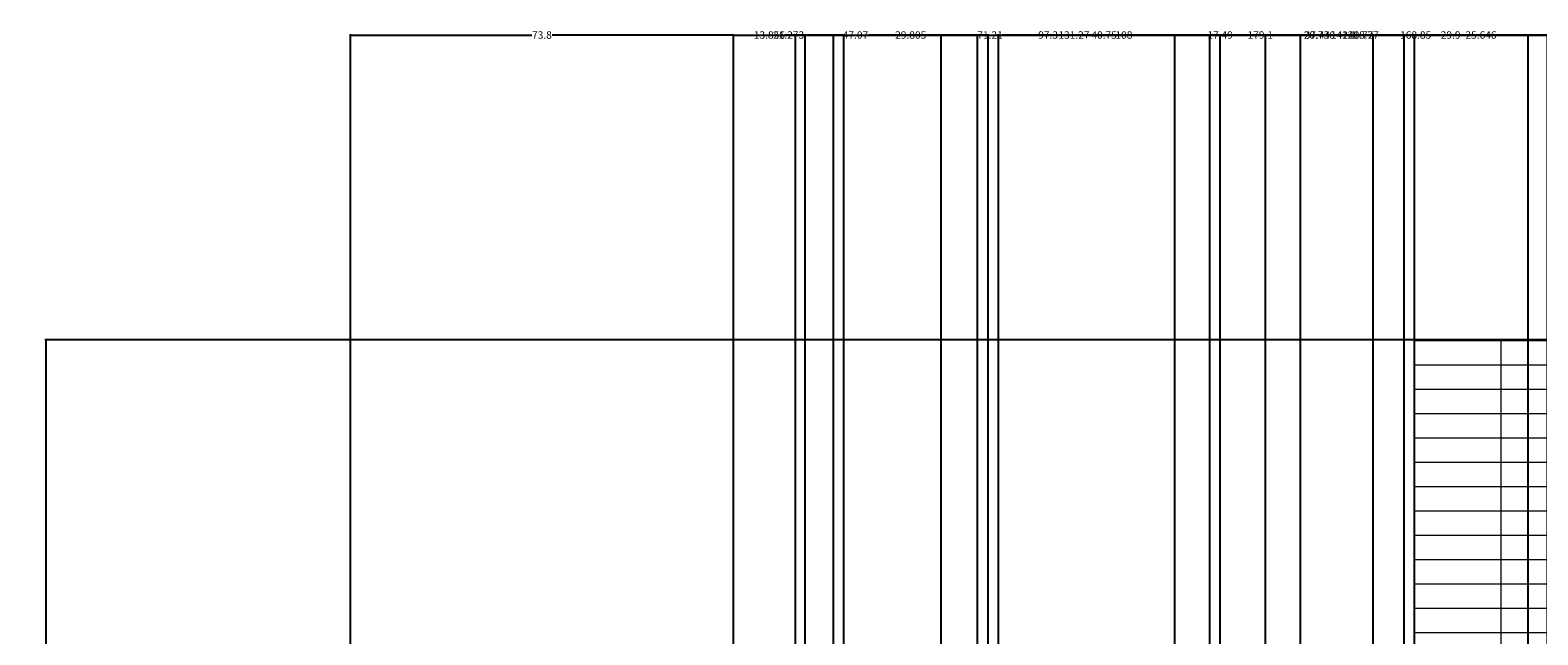
# Model space of a CAD drawing. Units: inches. Extents: x 241 to 943, y 109 to 1396.
# Tile 25 of 34: x 241 to 532, y 1279 to 1396. Entities that reach past the tile are written whole.
import ezdxf

# ---------------------------------------------------------------- set-up
doc = ezdxf.new("R2010")
doc.units = ezdxf.units.IN
doc.header["$MEASUREMENT"] = 0
for name, color, linetype, lineweight in [('A-ANNO-DIMS', 2, 'Continuous', 18), ('A-ELEV', 7, 'Continuous', 25), ('A-WALL-PATT', 8, 'Continuous', 13)]:
    doc.layers.add(name, color=color, linetype=linetype, lineweight=lineweight)
doc.styles.get("Standard").update_dxf_attribs({"font": 'arial.ttf'})
doc.dimstyles.get("Standard").update_dxf_attribs({"dimtxt": 1.4375, "dimasz": 0.18, "dimexe": 0.18, "dimexo": 0.0625, "dimgap": 0.09, "dimtad": 0, "dimtih": 1, "dimtoh": 1, "dimdec": 4, "dimzin": 0, "dimdsep": 46, "dimlunit": 4, "dimtxsty": 'Standard', "dimcen": 0.09, "dimadec": 0, "dimazin": 0, "dimtfac": 1, "dimtdec": 4, "dimtofl": 0, "dimtmove": 0, "dimatfit": 3, "dimfxl": 1, "dimtolj": 1, "dimtzin": 0, "dimarcsym": 0})

# ---------------------------------------------------------------- blocks, each defined once
blk = doc.blocks.new('*D5')
at = {"layer": 'A-ANNO-DIMS', "color": 0, "lineweight": -2, "transparency": 16777216}
for p, q in [((303.24, 177.8), (303.24, 1395.05)), ((377.04, 177.76), (377.04, 1395.05)), ((303.42, 1394.87), (338.18, 1394.87)), ((376.86, 1394.87), (342.09, 1394.87))]:
    blk.add_line(p, q, dxfattribs=at)
at = {"layer": 'A-ANNO-DIMS', "color": 0, "transparency": 16777216}
for points in [[(303.42, 1394.9), (303.42, 1394.84), (303.24, 1394.87)], [(376.86, 1394.9), (376.86, 1394.84), (377.04, 1394.87)]]:
    blk.add_solid(points, dxfattribs=at)
at = {"layer": 'Defpoints', "color": 0, "transparency": 16777216}
for p in [(377.04, 1394.87), (303.24, 177.74), (377.04, 177.7)]:
    blk.add_point(p, dxfattribs=at)
at = {"layer": 'A-ANNO-DIMS', "color": 0, "transparency": 16777216, "insert": (340.14, 1394.87), "char_height": 1.438, "attachment_point": 5}
blk.add_mtext('\\A1;73.8', dxfattribs=at)
blk = doc.blocks.new('*D7')
at = {"layer": 'A-ANNO-DIMS', "color": 0, "lineweight": -2, "transparency": 16777216}
for p, q in [((508.24, 1336.12), (244.31, 1336.12)), ((244.49, 1335.94), (244.49, 753.25)), ((244.49, 168.92), (244.49, 751.6)), ((303.17, 168.74), (244.31, 168.74))]:
    blk.add_line(p, q, dxfattribs=at)
at = {"layer": 'A-ANNO-DIMS', "color": 0, "transparency": 16777216}
for points in [[(244.46, 1335.94), (244.52, 1335.94), (244.49, 1336.12)], [(244.46, 168.92), (244.52, 168.92), (244.49, 168.74)]]:
    blk.add_solid(points, dxfattribs=at)
at = {"layer": 'Defpoints', "color": 0, "transparency": 16777216}
for p in [(244.49, 1336.12), (508.31, 1336.12), (303.24, 168.74)]:
    blk.add_point(p, dxfattribs=at)
at = {"layer": 'A-ANNO-DIMS', "color": 0, "transparency": 16777216, "insert": (244.49, 752.43), "char_height": 1.438, "attachment_point": 5}
blk.add_mtext('\\A1;1167.4', dxfattribs=at)
blk = doc.blocks.new('*D8')
at = {"layer": 'A-ANNO-DIMS', "color": 0, "lineweight": -2, "transparency": 16777216}
for p, q in [((377.04, 396.94), (377.04, 1395.05)), ((390.89, 384.24), (390.89, 1395.05)), ((377.22, 1394.87), (380.96, 1394.87)), ((390.71, 1394.87), (386.97, 1394.87))]:
    blk.add_line(p, q, dxfattribs=at)
at = {"layer": 'A-ANNO-DIMS', "color": 0, "transparency": 16777216}
for points in [[(377.22, 1394.9), (377.22, 1394.84), (377.04, 1394.87)], [(390.71, 1394.9), (390.71, 1394.84), (390.89, 1394.87)]]:
    blk.add_solid(points, dxfattribs=at)
at = {"layer": 'Defpoints', "color": 0, "transparency": 16777216}
for p in [(390.89, 1394.87), (377.04, 396.88), (390.89, 384.18)]:
    blk.add_point(p, dxfattribs=at)
at = {"layer": 'A-ANNO-DIMS', "color": 0, "transparency": 16777216, "insert": (383.97, 1394.87), "char_height": 1.438, "attachment_point": 5}
blk.add_mtext('\\A1;13.856', dxfattribs=at)
blk = doc.blocks.new('*D9')
at = {"layer": 'A-ANNO-DIMS', "color": 0, "lineweight": -2, "transparency": 16777216}
for p, q in [((390.89, 384.24), (390.89, 1395.05)), ((462.11, 384.24), (462.11, 1395.05)), ((391.07, 1394.87), (424.13, 1394.87)), ((461.93, 1394.87), (428.87, 1394.87))]:
    blk.add_line(p, q, dxfattribs=at)
at = {"layer": 'A-ANNO-DIMS', "color": 0, "transparency": 16777216}
for points in [[(391.07, 1394.9), (391.07, 1394.84), (390.89, 1394.87)], [(461.93, 1394.9), (461.93, 1394.84), (462.11, 1394.87)]]:
    blk.add_solid(points, dxfattribs=at)
at = {"layer": 'Defpoints', "color": 0, "transparency": 16777216}
for p in [(462.11, 1394.87), (390.89, 384.18), (462.11, 384.18)]:
    blk.add_point(p, dxfattribs=at)
at = {"layer": 'A-ANNO-DIMS', "color": 0, "transparency": 16777216, "insert": (426.5, 1394.87), "char_height": 1.438, "attachment_point": 5}
blk.add_mtext('\\A1;71.21', dxfattribs=at)
blk = doc.blocks.new('*D10')
at = {"layer": 'A-ANNO-DIMS', "color": 0, "lineweight": -2, "transparency": 16777216}
for p, q in [((462.11, 384.24), (462.11, 1395.05)), ((479.6, 384.24), (479.6, 1395.05)), ((462.29, 1394.87), (468.4, 1394.87)), ((479.42, 1394.87), (473.3, 1394.87))]:
    blk.add_line(p, q, dxfattribs=at)
at = {"layer": 'A-ANNO-DIMS', "color": 0, "transparency": 16777216}
for points in [[(462.29, 1394.9), (462.29, 1394.84), (462.11, 1394.87)], [(479.42, 1394.9), (479.42, 1394.84), (479.6, 1394.87)]]:
    blk.add_solid(points, dxfattribs=at)
at = {"layer": 'Defpoints', "color": 0, "transparency": 16777216}
for p in [(479.6, 1394.87), (462.11, 384.18), (479.6, 384.18)]:
    blk.add_point(p, dxfattribs=at)
at = {"layer": 'A-ANNO-DIMS', "color": 0, "transparency": 16777216, "insert": (470.85, 1394.87), "char_height": 1.438, "attachment_point": 5}
blk.add_mtext('\\A1;17.49', dxfattribs=at)
blk = doc.blocks.new('*D11')
at = {"layer": 'A-ANNO-DIMS', "color": 0, "lineweight": -2, "transparency": 16777216}
for p, q in [((500.33, 384.24), (500.33, 1395.05)), ((530.23, 384.24), (530.23, 1395.05)), ((500.51, 1394.87), (513.31, 1394.87)), ((530.05, 1394.87), (517.25, 1394.87))]:
    blk.add_line(p, q, dxfattribs=at)
at = {"layer": 'A-ANNO-DIMS', "color": 0, "transparency": 16777216}
for points in [[(500.51, 1394.9), (500.51, 1394.84), (500.33, 1394.87)], [(530.05, 1394.9), (530.05, 1394.84), (530.23, 1394.87)]]:
    blk.add_solid(points, dxfattribs=at)
at = {"layer": 'Defpoints', "color": 0, "transparency": 16777216}
for p in [(530.23, 1394.87), (500.33, 384.18), (530.23, 384.18)]:
    blk.add_point(p, dxfattribs=at)
at = {"layer": 'A-ANNO-DIMS', "color": 0, "transparency": 16777216, "insert": (515.28, 1394.87), "char_height": 1.438, "attachment_point": 5}
blk.add_mtext('\\A1;29.9', dxfattribs=at)
blk = doc.blocks.new('*D12')
at = {"layer": 'A-ANNO-DIMS', "color": 0, "lineweight": -2, "transparency": 16777216}
for p, q in [((530.23, 384.24), (530.23, 1395.05)), ((650.91, 384.24), (650.91, 1395.05)), ((530.41, 1394.87), (587.56, 1394.87)), ((650.73, 1394.87), (593.58, 1394.87))]:
    blk.add_line(p, q, dxfattribs=at)
at = {"layer": 'A-ANNO-DIMS', "color": 0, "transparency": 16777216}
for points in [[(530.41, 1394.9), (530.41, 1394.84), (530.23, 1394.87)], [(650.73, 1394.9), (650.73, 1394.84), (650.91, 1394.87)]]:
    blk.add_solid(points, dxfattribs=at)
at = {"layer": 'Defpoints', "color": 0, "transparency": 16777216}
for p in [(650.91, 1394.87), (530.23, 384.18), (650.91, 384.18)]:
    blk.add_point(p, dxfattribs=at)
at = {"layer": 'A-ANNO-DIMS', "color": 0, "transparency": 16777216, "insert": (590.57, 1394.87), "char_height": 1.438, "attachment_point": 5}
blk.add_mtext('\\A1;120.68', dxfattribs=at)
blk = doc.blocks.new('*D17')
at = {"layer": 'A-ANNO-DIMS', "color": 0, "lineweight": -2, "transparency": 16777216}
for p, q in [((377.04, 1275.98), (377.04, 1395.05)), ((508.31, 1275.98), (508.31, 1395.05)), ((377.22, 1394.87), (439.67, 1394.87)), ((508.13, 1394.87), (445.68, 1394.87))]:
    blk.add_line(p, q, dxfattribs=at)
at = {"layer": 'A-ANNO-DIMS', "color": 0, "transparency": 16777216}
for points in [[(377.22, 1394.9), (377.22, 1394.84), (377.04, 1394.87)], [(508.13, 1394.9), (508.13, 1394.84), (508.31, 1394.87)]]:
    blk.add_solid(points, dxfattribs=at)
at = {"layer": 'Defpoints', "color": 0, "transparency": 16777216}
for p in [(508.31, 1394.87), (377.04, 1275.91), (508.31, 1275.91)]:
    blk.add_point(p, dxfattribs=at)
at = {"layer": 'A-ANNO-DIMS', "color": 0, "transparency": 16777216, "insert": (442.67, 1394.87), "char_height": 1.438, "attachment_point": 5}
blk.add_mtext('\\A1;131.27', dxfattribs=at)
blk = doc.blocks.new('*D18')
at = {"layer": 'A-ANNO-DIMS', "color": 0, "lineweight": -2, "transparency": 16777216}
for p, q in [((508.31, 1336.18), (508.31, 1395.05)), ((747.76, 1336.18), (747.76, 1395.05)), ((508.49, 1394.87), (624.94, 1394.87)), ((747.58, 1394.87), (631.12, 1394.87))]:
    blk.add_line(p, q, dxfattribs=at)
at = {"layer": 'A-ANNO-DIMS', "color": 0, "transparency": 16777216}
for points in [[(508.49, 1394.9), (508.49, 1394.84), (508.31, 1394.87)], [(747.58, 1394.9), (747.58, 1394.84), (747.76, 1394.87)]]:
    blk.add_solid(points, dxfattribs=at)
at = {"layer": 'Defpoints', "color": 0, "transparency": 16777216}
for p in [(747.76, 1394.87), (508.31, 1336.12), (747.76, 1336.12)]:
    blk.add_point(p, dxfattribs=at)
at = {"layer": 'A-ANNO-DIMS', "color": 0, "transparency": 16777216, "insert": (628.03, 1394.87), "char_height": 1.438, "attachment_point": 5}
blk.add_mtext('\\A1;239.45', dxfattribs=at)
blk = doc.blocks.new('*D57')
at = {"layer": 'A-ANNO-DIMS', "color": 0, "lineweight": -2, "transparency": 16777216}
for p, q in [((508.31, 1070.92), (508.31, 1395.05)), ((533.95, 1108.23), (533.95, 1395.05)), ((508.49, 1394.87), (518.04, 1394.87)), ((533.77, 1394.87), (524.21, 1394.87))]:
    blk.add_line(p, q, dxfattribs=at)
at = {"layer": 'A-ANNO-DIMS', "color": 0, "transparency": 16777216}
for points in [[(508.49, 1394.9), (508.49, 1394.84), (508.31, 1394.87)], [(533.77, 1394.9), (533.77, 1394.84), (533.95, 1394.87)]]:
    blk.add_solid(points, dxfattribs=at)
at = {"layer": 'Defpoints', "color": 0, "transparency": 16777216}
for p in [(533.95, 1394.87), (533.95, 1108.17), (508.31, 1070.85)]:
    blk.add_point(p, dxfattribs=at)
at = {"layer": 'A-ANNO-DIMS', "color": 0, "transparency": 16777216, "insert": (521.13, 1394.87), "char_height": 1.438, "attachment_point": 5}
blk.add_mtext('\\A1;25.646', dxfattribs=at)
blk = doc.blocks.new('*D59')
at = {"layer": 'A-ANNO-DIMS', "color": 0, "lineweight": -2, "transparency": 16777216}
for p, q in [((398.31, 1175.6), (398.31, 1395.05)), ((506.31, 1175.6), (506.31, 1395.05)), ((398.49, 1394.87), (450.7, 1394.87)), ((506.13, 1394.87), (453.92, 1394.87))]:
    blk.add_line(p, q, dxfattribs=at)
at = {"layer": 'A-ANNO-DIMS', "color": 0, "transparency": 16777216}
for points in [[(398.49, 1394.9), (398.49, 1394.84), (398.31, 1394.87)], [(506.13, 1394.9), (506.13, 1394.84), (506.31, 1394.87)]]:
    blk.add_solid(points, dxfattribs=at)
at = {"layer": 'Defpoints', "color": 0, "transparency": 16777216}
for p in [(506.31, 1394.87), (398.31, 1175.54), (506.31, 1175.54)]:
    blk.add_point(p, dxfattribs=at)
at = {"layer": 'A-ANNO-DIMS', "color": 0, "transparency": 16777216, "insert": (452.31, 1394.87), "char_height": 1.438, "attachment_point": 5}
blk.add_mtext('\\A1;108', dxfattribs=at)
blk = doc.blocks.new('*D60')
at = {"layer": 'A-ANNO-DIMS', "color": 0, "lineweight": -2, "transparency": 16777216}
for p, q in [((377.04, 1177.6), (377.04, 1395.05)), ((398.31, 1175.6), (398.31, 1395.05)), ((377.22, 1394.87), (384.59, 1394.87)), ((398.13, 1394.87), (390.76, 1394.87))]:
    blk.add_line(p, q, dxfattribs=at)
at = {"layer": 'A-ANNO-DIMS', "color": 0, "transparency": 16777216}
for points in [[(377.22, 1394.9), (377.22, 1394.84), (377.04, 1394.87)], [(398.13, 1394.9), (398.13, 1394.84), (398.31, 1394.87)]]:
    blk.add_solid(points, dxfattribs=at)
at = {"layer": 'Defpoints', "color": 0, "transparency": 16777216}
for p in [(398.31, 1394.87), (377.04, 1177.54), (398.31, 1175.54)]:
    blk.add_point(p, dxfattribs=at)
at = {"layer": 'A-ANNO-DIMS', "color": 0, "transparency": 16777216, "insert": (387.68, 1394.87), "char_height": 1.438, "attachment_point": 5}
blk.add_mtext('\\A1;21.273', dxfattribs=at)
blk = doc.blocks.new('*D61')
at = {"layer": 'A-ANNO-DIMS', "color": 0, "lineweight": -2, "transparency": 16777216}
for p, q in [((377.04, 400.89), (377.04, 1395.05)), ((424.11, 568.89), (424.11, 1395.05)), ((377.22, 1394.87), (398.03, 1394.87)), ((423.93, 1394.87), (403.12, 1394.87))]:
    blk.add_line(p, q, dxfattribs=at)
at = {"layer": 'A-ANNO-DIMS', "color": 0, "transparency": 16777216}
for points in [[(377.22, 1394.9), (377.22, 1394.84), (377.04, 1394.87)], [(423.93, 1394.9), (423.93, 1394.84), (424.11, 1394.87)]]:
    blk.add_solid(points, dxfattribs=at)
at = {"layer": 'Defpoints', "color": 0, "transparency": 16777216}
for p in [(424.11, 1394.87), (424.11, 568.83), (377.04, 400.83)]:
    blk.add_point(p, dxfattribs=at)
at = {"layer": 'A-ANNO-DIMS', "color": 0, "transparency": 16777216, "insert": (400.57, 1394.87), "char_height": 1.438, "attachment_point": 5}
blk.add_mtext('\\A1;47.07', dxfattribs=at)
blk = doc.blocks.new('*D62')
at = {"layer": 'A-ANNO-DIMS', "color": 0, "lineweight": -2, "transparency": 16777216}
for p, q in [((424.11, 568.89), (424.11, 1395.05)), ((565.2, 568.89), (565.2, 1395.05)), ((424.29, 1394.87), (492.35, 1394.87)), ((565.02, 1394.87), (496.96, 1394.87))]:
    blk.add_line(p, q, dxfattribs=at)
at = {"layer": 'A-ANNO-DIMS', "color": 0, "transparency": 16777216}
for points in [[(424.29, 1394.9), (424.29, 1394.84), (424.11, 1394.87)], [(565.02, 1394.9), (565.02, 1394.84), (565.2, 1394.87)]]:
    blk.add_solid(points, dxfattribs=at)
at = {"layer": 'Defpoints', "color": 0, "transparency": 16777216}
for p in [(565.2, 1394.87), (424.11, 568.83), (565.2, 568.83)]:
    blk.add_point(p, dxfattribs=at)
at = {"layer": 'A-ANNO-DIMS', "color": 0, "transparency": 16777216, "insert": (494.66, 1394.87), "char_height": 1.438, "attachment_point": 5}
blk.add_mtext('\\A1;141.1', dxfattribs=at)
blk = doc.blocks.new('*D65')
at = {"layer": 'A-ANNO-DIMS', "color": 0, "lineweight": -2, "transparency": 16777216}
for p, q in [((424.11, 700.85), (424.11, 1395.05)), ((592.95, 700.85), (592.95, 1395.05)), ((424.29, 1394.87), (505.52, 1394.87)), ((592.77, 1394.87), (511.54, 1394.87))]:
    blk.add_line(p, q, dxfattribs=at)
at = {"layer": 'A-ANNO-DIMS', "color": 0, "transparency": 16777216}
for points in [[(424.29, 1394.9), (424.29, 1394.84), (424.11, 1394.87)], [(592.77, 1394.9), (592.77, 1394.84), (592.95, 1394.87)]]:
    blk.add_solid(points, dxfattribs=at)
at = {"layer": 'Defpoints', "color": 0, "transparency": 16777216}
for p in [(592.95, 1394.87), (424.11, 700.79), (592.95, 700.79)]:
    blk.add_point(p, dxfattribs=at)
at = {"layer": 'A-ANNO-DIMS', "color": 0, "transparency": 16777216, "insert": (508.53, 1394.87), "char_height": 1.438, "attachment_point": 5}
blk.add_mtext('\\A1;168.85', dxfattribs=at)
blk = doc.blocks.new('*D67')
at = {"layer": 'A-ANNO-DIMS', "color": 0, "lineweight": -2, "transparency": 16777216}
for p, q in [((389.04, 773.55), (389.04, 1395.05)), ((607.82, 773.55), (607.82, 1395.05)), ((389.22, 1394.87), (495.34, 1394.87)), ((607.64, 1394.87), (501.52, 1394.87))]:
    blk.add_line(p, q, dxfattribs=at)
at = {"layer": 'A-ANNO-DIMS', "color": 0, "transparency": 16777216}
for points in [[(389.22, 1394.9), (389.22, 1394.84), (389.04, 1394.87)], [(607.64, 1394.9), (607.64, 1394.84), (607.82, 1394.87)]]:
    blk.add_solid(points, dxfattribs=at)
at = {"layer": 'Defpoints', "color": 0, "transparency": 16777216}
for p in [(607.82, 1394.87), (389.04, 773.49), (607.82, 773.49)]:
    blk.add_point(p, dxfattribs=at)
at = {"layer": 'A-ANNO-DIMS', "color": 0, "transparency": 16777216, "insert": (498.43, 1394.87), "char_height": 1.438, "attachment_point": 5}
blk.add_mtext('\\A1;218.77', dxfattribs=at)
blk = doc.blocks.new('*D69')
at = {"layer": 'A-ANNO-DIMS', "color": 0, "lineweight": -2, "transparency": 16777216}
for p, q in [((389.04, 941.55), (389.04, 1395.05)), ((568.13, 941.55), (568.13, 1395.05)), ((389.22, 1394.87), (476.28, 1394.87)), ((567.95, 1394.87), (480.9, 1394.87))]:
    blk.add_line(p, q, dxfattribs=at)
at = {"layer": 'A-ANNO-DIMS', "color": 0, "transparency": 16777216}
for points in [[(389.22, 1394.9), (389.22, 1394.84), (389.04, 1394.87)], [(567.95, 1394.9), (567.95, 1394.84), (568.13, 1394.87)]]:
    blk.add_solid(points, dxfattribs=at)
at = {"layer": 'Defpoints', "color": 0, "transparency": 16777216}
for p in [(568.13, 1394.87), (389.04, 941.49), (568.13, 941.49)]:
    blk.add_point(p, dxfattribs=at)
at = {"layer": 'A-ANNO-DIMS', "color": 0, "transparency": 16777216, "insert": (478.59, 1394.87), "char_height": 1.438, "attachment_point": 5}
blk.add_mtext('\\A1;179.1', dxfattribs=at)
blk = doc.blocks.new('*D72')
at = {"layer": 'A-ANNO-DIMS', "color": 0, "lineweight": -2, "transparency": 16777216}
for p, q in [((389.04, 1109.55), (389.04, 1395.05)), ((486.34, 1109.55), (486.34, 1395.05)), ((389.22, 1394.87), (435.74, 1394.87)), ((486.16, 1394.87), (439.65, 1394.87))]:
    blk.add_line(p, q, dxfattribs=at)
at = {"layer": 'A-ANNO-DIMS', "color": 0, "transparency": 16777216}
for points in [[(389.22, 1394.9), (389.22, 1394.84), (389.04, 1394.87)], [(486.16, 1394.9), (486.16, 1394.84), (486.34, 1394.87)]]:
    blk.add_solid(points, dxfattribs=at)
at = {"layer": 'Defpoints', "color": 0, "transparency": 16777216}
for p in [(486.34, 1394.87), (389.04, 1109.49), (486.34, 1109.49)]:
    blk.add_point(p, dxfattribs=at)
at = {"layer": 'A-ANNO-DIMS', "color": 0, "transparency": 16777216, "insert": (437.69, 1394.87), "char_height": 1.438, "attachment_point": 5}
blk.add_mtext('\\A1;97.3', dxfattribs=at)
blk = doc.blocks.new('*D79')
at = {"layer": 'A-ANNO-DIMS', "color": 0, "lineweight": -2, "transparency": 16777216}
for p, q in [((479.6, 384.24), (479.6, 1395.05)), ((500.33, 384.24), (500.33, 1395.05)), ((479.78, 1394.87), (486.88, 1394.87)), ((500.15, 1394.87), (493.05, 1394.87))]:
    blk.add_line(p, q, dxfattribs=at)
at = {"layer": 'A-ANNO-DIMS', "color": 0, "transparency": 16777216}
for points in [[(479.78, 1394.9), (479.78, 1394.84), (479.6, 1394.87)], [(500.15, 1394.9), (500.15, 1394.84), (500.33, 1394.87)]]:
    blk.add_solid(points, dxfattribs=at)
at = {"layer": 'Defpoints', "color": 0, "transparency": 16777216}
for p in [(500.33, 1394.87), (479.6, 384.18), (500.33, 384.18)]:
    blk.add_point(p, dxfattribs=at)
at = {"layer": 'A-ANNO-DIMS', "color": 0, "transparency": 16777216, "insert": (489.96, 1394.87), "char_height": 1.438, "attachment_point": 5}
blk.add_mtext('\\A1;20.736', dxfattribs=at)
blk = doc.blocks.new('*D89')
at = {"layer": 'A-ANNO-DIMS', "color": 0, "lineweight": -2, "transparency": 16777216}
for p, q in [((377.04, 841.6), (377.04, 1395.05)), ((617.76, 841.6), (617.76, 1395.05)), ((377.22, 1394.87), (494.32, 1394.87)), ((617.58, 1394.87), (500.48, 1394.87))]:
    blk.add_line(p, q, dxfattribs=at)
at = {"layer": 'A-ANNO-DIMS', "color": 0, "transparency": 16777216}
for points in [[(377.22, 1394.9), (377.22, 1394.84), (377.04, 1394.87)], [(617.58, 1394.9), (617.58, 1394.84), (617.76, 1394.87)]]:
    blk.add_solid(points, dxfattribs=at)
at = {"layer": 'Defpoints', "color": 0, "transparency": 16777216}
for p in [(617.76, 1394.87), (377.04, 841.54), (617.76, 841.54)]:
    blk.add_point(p, dxfattribs=at)
at = {"layer": 'A-ANNO-DIMS', "color": 0, "transparency": 16777216, "insert": (497.4, 1394.87), "char_height": 1.438, "attachment_point": 5}
blk.add_mtext('\\A1;240.72', dxfattribs=at)
blk = doc.blocks.new('*D92')
at = {"layer": 'A-ANNO-DIMS', "color": 0, "lineweight": -2, "transparency": 16777216}
for p, q in [((508.24, 1336.12), (244.31, 1336.12)), ((244.49, 1335.94), (244.49, 1204.31)), ((244.49, 1071.03), (244.49, 1202.66)), ((508.24, 1070.85), (244.31, 1070.85))]:
    blk.add_line(p, q, dxfattribs=at)
at = {"layer": 'A-ANNO-DIMS', "color": 0, "transparency": 16777216}
for points in [[(244.46, 1335.94), (244.52, 1335.94), (244.49, 1336.12)], [(244.46, 1071.03), (244.52, 1071.03), (244.49, 1070.85)]]:
    blk.add_solid(points, dxfattribs=at)
at = {"layer": 'Defpoints', "color": 0, "transparency": 16777216}
for p in [(244.49, 1336.12), (508.31, 1336.12), (508.31, 1070.85)]:
    blk.add_point(p, dxfattribs=at)
at = {"layer": 'A-ANNO-DIMS', "color": 0, "transparency": 16777216, "insert": (244.49, 1203.48), "char_height": 1.438, "attachment_point": 5}
blk.add_mtext('\\A1;265.26', dxfattribs=at)
blk = doc.blocks.new('*D99')
at = {"layer": 'A-ANNO-DIMS', "color": 0, "lineweight": -2, "transparency": 16777216}
for p, q in [((417.09, 181.71), (417.09, 1395.05)), ((667.39, 214.58), (667.39, 1395.05)), ((417.27, 1394.87), (539.16, 1394.87)), ((667.21, 1394.87), (545.33, 1394.87))]:
    blk.add_line(p, q, dxfattribs=at)
at = {"layer": 'A-ANNO-DIMS', "color": 0, "transparency": 16777216}
for points in [[(417.27, 1394.9), (417.27, 1394.84), (417.09, 1394.87)], [(667.21, 1394.9), (667.21, 1394.84), (667.39, 1394.87)]]:
    blk.add_solid(points, dxfattribs=at)
at = {"layer": 'Defpoints', "color": 0, "transparency": 16777216}
for p in [(667.39, 1394.87), (667.39, 214.52), (417.09, 181.65)]:
    blk.add_point(p, dxfattribs=at)
at = {"layer": 'A-ANNO-DIMS', "color": 0, "transparency": 16777216, "insert": (542.24, 1394.87), "char_height": 1.438, "attachment_point": 5}
blk.add_mtext('\\A1;250.30', dxfattribs=at)
blk = doc.blocks.new('*D101')
at = {"layer": 'A-ANNO-DIMS', "color": 0, "lineweight": -2, "transparency": 16777216}
for p, q in [((396.31, 1009.6), (396.31, 1395.05)), ((426.12, 1007.6), (426.12, 1395.05)), ((396.49, 1394.87), (408.12, 1394.87)), ((425.94, 1394.87), (414.31, 1394.87))]:
    blk.add_line(p, q, dxfattribs=at)
at = {"layer": 'A-ANNO-DIMS', "color": 0, "transparency": 16777216}
for points in [[(396.49, 1394.9), (396.49, 1394.84), (396.31, 1394.87)], [(425.94, 1394.9), (425.94, 1394.84), (426.12, 1394.87)]]:
    blk.add_solid(points, dxfattribs=at)
at = {"layer": 'Defpoints', "color": 0, "transparency": 16777216}
for p in [(426.12, 1394.87), (396.31, 1009.54), (426.12, 1007.54)]:
    blk.add_point(p, dxfattribs=at)
at = {"layer": 'A-ANNO-DIMS', "color": 0, "transparency": 16777216, "insert": (411.21, 1394.87), "char_height": 1.438, "attachment_point": 5}
blk.add_mtext('\\A1;29.805', dxfattribs=at)
blk = doc.blocks.new('*D102')
at = {"layer": 'A-ANNO-DIMS', "color": 0, "lineweight": -2, "transparency": 16777216}
for p, q in [((428.12, 1007.6), (428.12, 1395.05)), ((468.87, 1007.6), (468.87, 1395.05)), ((428.3, 1394.87), (445.94, 1394.87)), ((468.69, 1394.87), (451.04, 1394.87))]:
    blk.add_line(p, q, dxfattribs=at)
at = {"layer": 'A-ANNO-DIMS', "color": 0, "transparency": 16777216}
for points in [[(428.3, 1394.9), (428.3, 1394.84), (428.12, 1394.87)], [(468.69, 1394.9), (468.69, 1394.84), (468.87, 1394.87)]]:
    blk.add_solid(points, dxfattribs=at)
at = {"layer": 'Defpoints', "color": 0, "transparency": 16777216}
for p in [(468.87, 1394.87), (428.12, 1007.54), (468.87, 1007.54)]:
    blk.add_point(p, dxfattribs=at)
at = {"layer": 'A-ANNO-DIMS', "color": 0, "transparency": 16777216, "insert": (448.49, 1394.87), "char_height": 1.438, "attachment_point": 5}
blk.add_mtext('\\A1;40.75', dxfattribs=at)
blk = doc.blocks.new('*D103')
at = {"layer": 'A-ANNO-DIMS', "color": 0, "lineweight": -2, "transparency": 16777216}
for p, q in [((470.87, 1007.6), (470.87, 1395.05)), ((508.31, 1009.6), (508.31, 1395.05)), ((471.05, 1394.87), (487.08, 1394.87)), ((508.13, 1394.87), (492.1, 1394.87))]:
    blk.add_line(p, q, dxfattribs=at)
at = {"layer": 'A-ANNO-DIMS', "color": 0, "transparency": 16777216}
for points in [[(471.05, 1394.9), (471.05, 1394.84), (470.87, 1394.87)], [(508.13, 1394.9), (508.13, 1394.84), (508.31, 1394.87)]]:
    blk.add_solid(points, dxfattribs=at)
at = {"layer": 'Defpoints', "color": 0, "transparency": 16777216}
for p in [(508.31, 1394.87), (508.31, 1009.54), (470.87, 1007.54)]:
    blk.add_point(p, dxfattribs=at)
at = {"layer": 'A-ANNO-DIMS', "color": 0, "transparency": 16777216, "insert": (489.59, 1394.87), "char_height": 1.438, "attachment_point": 5}
blk.add_mtext('\\A1;37.44', dxfattribs=at)

msp = doc.modelspace()

# ---------------------------------------------------------------- hatches: boundary and pattern name
at = {"layer": 'A-WALL-PATT'}
h = msp.add_hatch(dxfattribs=at)
h.set_pattern_fill('GRATE', color=256, scale=150)
h.paths.add_polyline_path([(747.7579, 1238.8538), (747.7579, 1275.9142), (747.7579, 1336.1154), (508.3064, 1336.1154), (508.3064, 1275.9142), (508.3064, 1238.8538), (508.3064, 1177.5382), (508.3064, 1109.4916), (508.3064, 1070.8538), (553.5166, 1070.8538), (749.6328, 1070.8538)])
h.paths.add_polyline_path([(533.952, 1108.1686), (533.952, 1177.7336), (533.952, 1303.0286), (724.819, 1303.0286), (724.819, 1108.1686)], flags=16)
h.paths.add_polyline_path([(535.952, 1110.1686), (535.952, 1175.7336), (722.819, 1175.7336), (722.819, 1110.1686)], flags=0)
h.paths.add_polyline_path([(643.4534, 1134.0739), (622.521, 1134.0739), (622.521, 1136.0739), (643.4534, 1136.0739)], flags=0)
h.paths.add_polyline_path([(617.7594, 568.8295), (617.7594, 734.8538), (377.0391, 734.8538), (377.0391, 566.8538), (377.0391, 400.8295), (417.0913, 400.8295), (618.9643, 400.8295)])
h.paths.add_polyline_path([(424.1086, 496.4395), (424.1086, 568.8295), (565.2023, 568.8295), (565.2023, 496.4395)], flags=16)
h.paths.add_polyline_path([(426.1086, 498.4395), (426.1086, 566.8295), (563.2023, 566.8295), (563.2023, 508.9074), (563.2023, 498.4395)], flags=0)
h.paths.add_polyline_path([(508.0803, 508.9074), (508.0803, 519.3754), (450.9259, 519.3754), (450.9259, 525.3816), (445.5808, 525.3816, -1), (445.5808, 527.3816), (450.9259, 527.3816), (450.9259, 566.8295), (508.0803, 566.8295), (537.4269, 566.8295), (537.4269, 508.9074)], flags=0)
h.paths.add_polyline_path([(506.0803, 521.3754), (452.9259, 521.3754), (452.9259, 564.8295), (506.0803, 564.8295)], flags=0)
h.paths.add_polyline_path([(424.1086, 628.4013), (424.1086, 700.7912), (592.9542, 700.7912), (592.9542, 628.4013)], flags=16)
h.paths.add_polyline_path([(426.1086, 630.4013), (426.1086, 698.7912), (590.8792, 698.7912), (590.8792, 630.4013)], flags=0)
h.paths.add_polyline_path([(508.1906, 651.3371), (508.0803, 651.3371), (450.9259, 651.3371), (428.0291, 651.3371), (428.0291, 698.7912), (451.9767, 698.7912), (508.0803, 698.7912), (537.4269, 698.7912), (563.2023, 698.7912), (563.2023, 659.3434), (563.9297, 659.3434), (563.9297, 651.3371)], flags=0)
h.paths.add_polyline_path([(506.0803, 653.3371), (452.9259, 653.3371), (452.9259, 657.3434), (445.5808, 657.3434, -1), (445.5808, 659.3434), (452.9259, 659.3434), (452.9259, 696.7912), (506.0803, 696.7912)], flags=0)

# ---------------------------------------------------------------- linework, layer by layer
at = {"layer": 'A-ELEV'}
for p in [(508.3064, 1275.9142), (747.7579, 1336.1154)]:
    msp.add_line(p, (508.3064, 1336.1154), dxfattribs=at)

# ---------------------------------------------------------------- dimensions: what is measured, and where the dimension line sits
at = {"layer": 'A-ANNO-DIMS'}
for base, p1, p2, override, picture, middle in [((377.0391, 1394.8654), (303.2358, 177.7407), (377.0391, 177.6977), {"dimdec": 1, "dimlfac": 1, "dimrnd": 0, "dimzin": 0, "dimdsep": 46, "dimlunit": 2}, '*D5', (340.1375, 1394.8654)), ((390.895, 1394.8654), (377.0391, 396.8782), (390.895, 384.1784), {"dimdec": 3, "dimlfac": 1, "dimrnd": 0, "dimzin": 0, "dimdsep": 46, "dimlunit": 2}, '*D8', (383.9671, 1394.8654)), ((508.3064, 1394.8654), (377.0391, 1275.9142), (508.3064, 1275.9142), {"dimdec": 2, "dimlfac": 1, "dimrnd": 0, "dimzin": 0, "dimdsep": 46, "dimlunit": 2}, '*D17', (442.6728, 1394.8654)), ((398.3125, 1394.8654), (377.0391, 1177.5382), (398.3125, 1175.5382), {"dimdec": 3, "dimlfac": 1, "dimrnd": 0, "dimzin": 0, "dimdsep": 46, "dimlunit": 2}, '*D60', (387.6758, 1394.8654)), ((424.1086, 1394.8654), (377.0391, 400.8295), (424.1086, 568.8295), {"dimdec": 2, "dimlfac": 1, "dimrnd": 0, "dimzin": 0, "dimdsep": 46, "dimlunit": 2}, '*D61', (400.5739, 1394.8654)), ((617.7594, 1394.8654), (377.0391, 841.5382), (617.7594, 841.5382), {"dimdec": 2, "dimlfac": 1, "dimrnd": 0, "dimzin": 0, "dimdsep": 46, "dimlunit": 2}, '*D89', (497.3993, 1394.8654)), ((607.8162, 1394.8654), (389.0429, 773.4916), (607.8162, 773.4916), {"dimdec": 2, "dimlfac": 1, "dimrnd": 0, "dimzin": 0, "dimdsep": 46, "dimlunit": 2}, '*D67', (498.4295, 1394.8654)), ((568.1348, 1394.8654), (389.0429, 941.4916), (568.1348, 941.4916), {"dimdec": 1, "dimlfac": 1, "dimrnd": 0, "dimzin": 0, "dimdsep": 46, "dimlunit": 2}, '*D69', (478.5888, 1394.8654)), ((486.3418, 1394.8654), (389.0429, 1109.4916), (486.3418, 1109.4916), {"dimdec": 1, "dimlfac": 1, "dimrnd": 0, "dimzin": 0, "dimdsep": 46, "dimlunit": 2}, '*D72', (437.6924, 1394.8654)), ((462.1074, 1394.8654), (390.895, 384.1784), (462.1074, 384.1784), {"dimdec": 2, "dimlfac": 1, "dimrnd": 0, "dimzin": 0, "dimdsep": 46, "dimlunit": 2}, '*D9', (426.5012, 1394.8654)), ((426.1173, 1394.8654), (396.3125, 1009.5382), (426.1173, 1007.5382), {"dimdec": 3, "dimlfac": 1, "dimrnd": 0, "dimzin": 0, "dimdsep": 46, "dimlunit": 2}, '*D101', (411.2149, 1394.8654)), ((506.3064, 1394.8654), (398.3125, 1175.5382), (506.3064, 1175.5382), {"dimdec": 0, "dimlfac": 1, "dimrnd": 0, "dimzin": 0, "dimdsep": 46, "dimlunit": 2}, '*D59', (452.3095, 1394.8654)), ((667.3935, 1394.8654), (417.0913, 181.649), (667.3935, 214.5189), {"dimdec": 2, "dimlfac": 1, "dimrnd": 0, "dimzin": 0, "dimdsep": 46, "dimlunit": 2}, '*D99', (542.2424, 1394.8654)), ((565.2023, 1394.8654), (424.1086, 568.8295), (565.2023, 568.8295), {"dimdec": 1, "dimlfac": 1, "dimrnd": 0, "dimzin": 0, "dimdsep": 46, "dimlunit": 2}, '*D62', (494.6554, 1394.8654)), ((592.9542, 1394.8654), (424.1086, 700.7912), (592.9542, 700.7912), {"dimdec": 2, "dimlfac": 1, "dimrnd": 0, "dimzin": 0, "dimdsep": 46, "dimlunit": 2}, '*D65', (508.5314, 1394.8654)), ((468.8692, 1394.8654), (428.1173, 1007.5382), (468.8692, 1007.5382), {"dimdec": 2, "dimlfac": 1, "dimrnd": 0, "dimzin": 0, "dimdsep": 46, "dimlunit": 2}, '*D102', (448.4933, 1394.8654)), ((479.596, 1394.8654), (462.1074, 384.1784), (479.596, 384.1784), {"dimdec": 2, "dimlfac": 1, "dimrnd": 0, "dimzin": 0, "dimdsep": 46, "dimlunit": 2}, '*D10', (470.8517, 1394.8654)), ((508.3064, 1394.8654), (470.8692, 1007.5382), (508.3064, 1009.5382), {"dimdec": 2, "dimlfac": 1, "dimrnd": 0, "dimzin": 0, "dimdsep": 46, "dimlunit": 2}, '*D103', (489.5878, 1394.8654)), ((500.3323, 1394.8654), (479.596, 384.1784), (500.3323, 384.1784), {"dimdec": 3, "dimlfac": 1, "dimrnd": 0, "dimzin": 0, "dimdsep": 46, "dimlunit": 2}, '*D79', (489.9641, 1394.8654)), ((530.2303, 1394.8654), (500.3323, 384.1784), (530.2303, 384.1784), {"dimdec": 1, "dimlfac": 1, "dimrnd": 0, "dimzin": 0, "dimdsep": 46, "dimlunit": 2}, '*D11', (515.2813, 1394.8654)), ((747.7579, 1394.8654), (508.3064, 1336.1154), (747.7579, 1336.1154), {"dimdec": 2, "dimlfac": 1, "dimrnd": 0, "dimzin": 0, "dimdsep": 46, "dimlunit": 2}, '*D18', (628.0322, 1394.8654)), ((533.952, 1394.8654), (508.3064, 1070.8538), (533.952, 1108.1686), {"dimdec": 3, "dimlfac": 1, "dimrnd": 0, "dimzin": 0, "dimdsep": 46, "dimlunit": 2}, '*D57', (521.1292, 1394.8654)), ((650.907, 1394.8654), (530.2303, 384.1784), (650.907, 384.1784), {"dimdec": 2, "dimlfac": 1, "dimrnd": 0, "dimzin": 0, "dimdsep": 46, "dimlunit": 2}, '*D12', (590.5686, 1394.8654))]:
    dim = msp.add_linear_dim(base=base, p1=p1, p2=p2, dimstyle='Standard', override=override, dxfattribs=at)
    dim.commit()
    dim.dimension.update_dxf_attribs({"geometry": picture, "text_midpoint": middle})
for p1, override, picture, middle in [((303.2358, 168.7407), {"dimdec": 1, "dimlfac": 1, "dimrnd": 0, "dimzin": 0, "dimdsep": 46, "dimlunit": 2}, '*D7', (244.4858, 752.4281)), ((508.3064, 1070.8538), {"dimdec": 2, "dimlfac": 1, "dimrnd": 0, "dimzin": 0, "dimdsep": 46, "dimlunit": 2}, '*D92', (244.4858, 1203.4846))]:
    dim = msp.add_linear_dim(base=(244.4858, 1336.1154), p1=p1, p2=(508.3064, 1336.1154), angle=90, dimstyle='Standard', override=override, dxfattribs=at)
    dim.commit()
    dim.dimension.update_dxf_attribs({"geometry": picture, "text_midpoint": middle})

doc.saveas('drawing.dxf')
